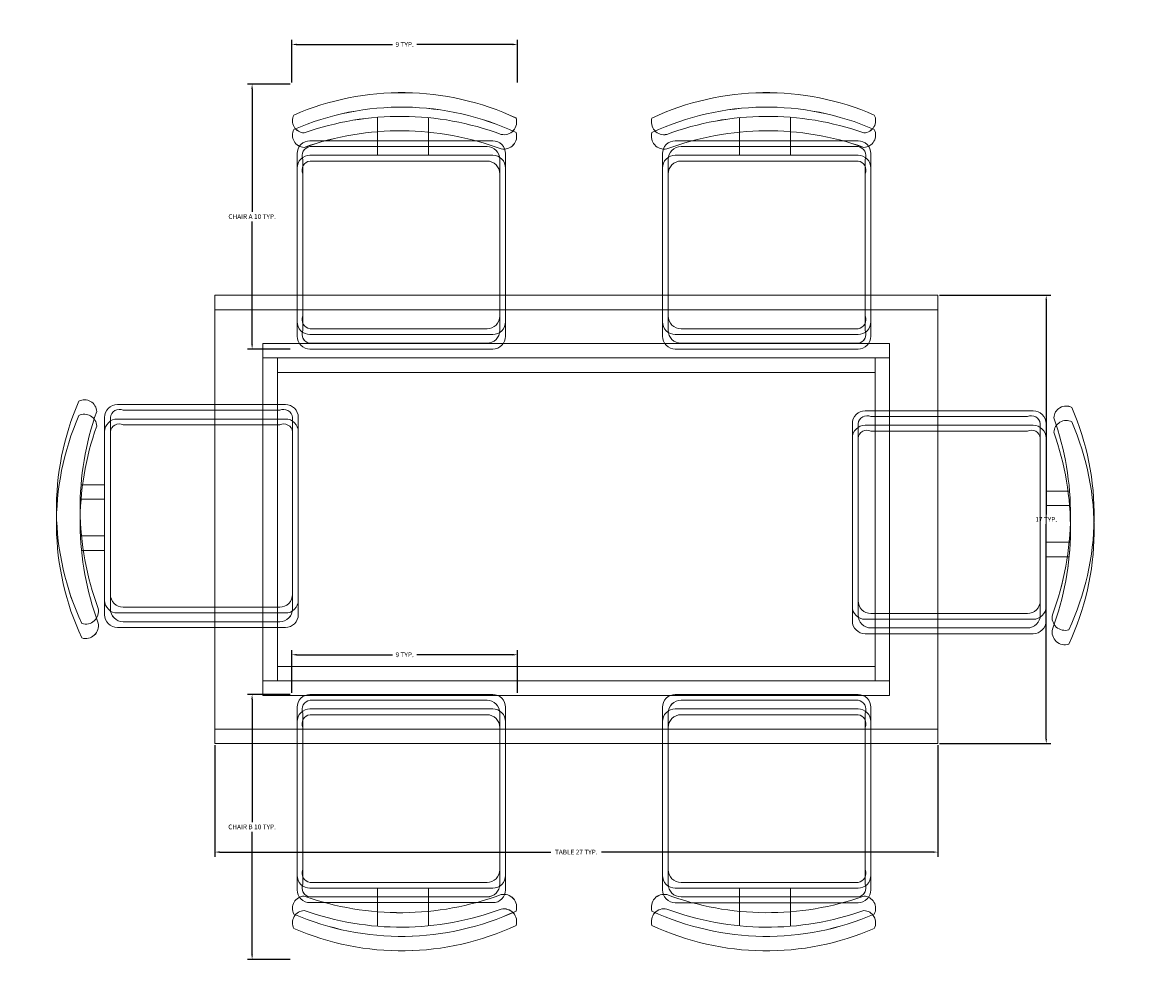
# Model space of a CAD drawing. Units: inches. Extents: x 2163 to 2982, y 1024 to 2288.
# Tile 14 of 22: x 2490 to 2532, y 1920 to 1957. Entities that reach past the tile are written whole.
import ezdxf

# ---------------------------------------------------------------- set-up
doc = ezdxf.new("R2010")
doc.units = ezdxf.units.IN
doc.layers.add('A-ANNO-DIMS', color=2, linetype='Continuous', lineweight=18)
doc.layers.add('A-FURN', color=8, linetype='Continuous', lineweight=13)
doc.styles.get("Standard").update_dxf_attribs({"font": 'arial.ttf'})
doc.dimstyles.get("Standard").update_dxf_attribs({"dimtxt": 0.18, "dimasz": 0.18, "dimexe": 0.18, "dimexo": 0.0625, "dimgap": 0.09, "dimtad": 0, "dimtih": 1, "dimtoh": 1, "dimdec": 4, "dimzin": 0, "dimdsep": 46, "dimtxsty": 'Standard', "dimcen": 0.09, "dimadec": 0, "dimazin": 0, "dimtfac": 1, "dimtdec": 4, "dimtofl": 0, "dimtmove": 0, "dimatfit": 3, "dimfxl": 1, "dimtolj": 1, "dimtzin": 0, "dimarcsym": 0})

# ---------------------------------------------------------------- blocks, each defined once
blk = doc.blocks.new('TABLE-DINING')
for points in [[(0, 17.017), (27.445, 17.017), (27.445, 0.549), (0, 0.549)], [(0, 17.017), (27.445, 17.017), (27.445, 0.549), (0, 0.549)], [(0, 17.016), (27.445, 17.016), (27.445, 0.549), (0, 0.549)], [(0, 17.016), (27.445, 17.016), (27.445, 0.549), (0, 0.549)], [(0, 16.468), (27.445, 16.468), (27.445, 0), (0, 0)], [(0, 16.468), (27.445, 16.468), (27.445, 0), (0, 0)], [(0, 16.467), (27.445, 16.467), (27.445, 0), (0, 0)], [(0, 16.467), (27.445, 16.467), (27.445, 0), (0, 0)], [(1.829, 15.187), (25.616, 15.187), (25.616, 2.379), (1.829, 2.379)], [(1.829, 15.187), (25.616, 15.187), (25.616, 2.379), (1.829, 2.379)], [(1.829, 15.187), (25.616, 15.187), (25.616, 2.379), (1.829, 2.379)], [(1.829, 15.187), (25.616, 15.187), (25.616, 2.379), (1.829, 2.379)], [(1.829, 14.638), (25.616, 14.638), (25.616, 1.83), (1.829, 1.83)], [(1.829, 14.638), (25.616, 14.638), (25.616, 1.83), (1.829, 1.83)], [(1.829, 14.638), (25.616, 14.638), (25.616, 1.83), (1.829, 1.83)], [(1.829, 14.638), (25.616, 14.638), (25.616, 1.83), (1.829, 1.83)], [(2.378, 14.638), (25.067, 14.638), (25.067, 2.928), (2.378, 2.928)], [(2.378, 14.638), (25.067, 14.638), (25.067, 2.927), (2.378, 2.927)], [(2.378, 14.638), (25.067, 14.638), (25.067, 2.928), (2.378, 2.928)], [(2.378, 14.638), (25.067, 14.638), (25.067, 2.927), (2.378, 2.927)], [(2.378, 14.089), (25.067, 14.089), (25.067, 2.379), (2.378, 2.379)], [(2.378, 14.089), (25.067, 14.089), (25.067, 2.379), (2.378, 2.379)], [(2.378, 14.089), (25.067, 14.089), (25.067, 2.379), (2.378, 2.379)], [(2.378, 14.089), (25.067, 14.089), (25.067, 2.379), (2.378, 2.379)]]:
    blk.add_lwpolyline(points, close=True)
blk = doc.blocks.new('CHAIR-DINING-A')
for points in [[(0.449, 8.202, -0.175809), (7.925, 8.145, 0.578392), (8.491, 8.768, 0.214524), (0.053, 8.881, 0.552014), (0.449, 8.202, -0.065079)], [(0.449, 8.201, -0.175809), (7.925, 8.145, 0.578392), (8.491, 8.767, 0.214524), (0.053, 8.881, 0.552014), (0.449, 8.201, -0.065079)], [(0.449, 8.202, -0.175809), (7.925, 8.145, 0.578392), (8.491, 8.768, 0.214524), (0.053, 8.881, 0.552014), (0.449, 8.202, -0.065079)], [(0.449, 8.201, -0.175809), (7.925, 8.145, 0.578392), (8.491, 8.767, 0.214524), (0.053, 8.881, 0.552014), (0.449, 8.201, -0.065079)], [(0.449, 7.653, -0.175809), (7.925, 7.596, 0.578392), (8.491, 8.219, 0.214524), (0.053, 8.332, 0.552014), (0.449, 7.653, -0.065079)], [(0.449, 7.652, -0.175809), (7.925, 7.596, 0.578392), (8.491, 8.218, 0.214524), (0.053, 8.332, 0.552014), (0.449, 7.652, -0.065079)], [(0.449, 7.653, -0.175809), (7.925, 7.596, 0.578392), (8.491, 8.219, 0.214524), (0.053, 8.332, 0.552014), (0.449, 7.653, -0.065079)], [(0.449, 7.652, -0.175809), (7.925, 7.596, 0.578392), (8.491, 8.218, 0.214524), (0.053, 8.332, 0.552014), (0.449, 7.652, -0.065079)], [(5.17, 7.902), (5.17, 8.779, -0.064759)], [(5.17, 7.901), (5.17, 8.779, -0.064759)], [(5.17, 7.902), (5.17, 8.779, -0.064759)], [(5.17, 7.901), (5.17, 8.779, -0.064759)], [(5.17, 7.353), (5.17, 8.23, -0.064759)], [(5.17, 7.352), (5.17, 8.23, -0.064759)], [(5.17, 7.353), (5.17, 8.23, -0.064759)], [(5.17, 7.352), (5.17, 8.23, -0.064759)], [(7.608, 7.902), (0.668, 7.902, 0.414214), (0.182, 7.416), (0.182, 1.035, 0.414214), (0.668, 0.549), (7.608, 0.549, 0.414214), (8.093, 1.035), (8.093, 7.416, 0.414214), (7.608, 7.902)], [(7.608, 7.902), (0.668, 7.902, 0.414214), (0.182, 7.416), (0.182, 1.035, 0.414214), (0.668, 0.549), (7.608, 0.549, 0.414214), (8.093, 1.035), (8.093, 7.416, 0.414214), (7.608, 7.902)], [(7.608, 7.901), (0.668, 7.901, 0.414214), (0.182, 7.416), (0.182, 1.035, 0.414214), (0.668, 0.549), (7.608, 0.549, 0.414214), (8.093, 1.035), (8.093, 7.416, 0.414214), (7.608, 7.901)], [(7.608, 7.901), (0.668, 7.901, 0.414214), (0.182, 7.416), (0.182, 1.035, 0.414214), (0.668, 0.549), (7.608, 0.549, 0.414214), (8.093, 1.035), (8.093, 7.416, 0.414214), (7.608, 7.901)], [(7.608, 7.353), (0.668, 7.353, 0.414214), (0.182, 6.867), (0.182, 0.486, 0.414214), (0.668, 0), (7.608, 0, 0.414214), (8.093, 0.486), (8.093, 6.867, 0.414214), (7.608, 7.353)], [(7.608, 7.353), (0.668, 7.353, 0.414214), (0.182, 6.867), (0.182, 0.486, 0.414214), (0.668, 0), (7.608, 0, 0.414214), (8.093, 0.486), (8.093, 6.867, 0.414214), (7.608, 7.353)], [(7.608, 7.352), (0.668, 7.352, 0.414214), (0.182, 6.867), (0.182, 0.486, 0.414214), (0.668, 0), (7.608, 0, 0.414214), (8.093, 0.486), (8.093, 6.867, 0.414214), (7.608, 7.352)], [(7.608, 7.352), (0.668, 7.352, 0.414214), (0.182, 6.867), (0.182, 0.486, 0.414214), (0.668, 0), (7.608, 0, 0.414214), (8.093, 0.486), (8.093, 6.867, 0.414214), (7.608, 7.352)]]:
    blk.add_lwpolyline(points, format="xyb")
for points in [[(3.227, 8.795), (3.227, 7.902)], [(3.227, 8.795), (3.227, 7.901)], [(3.227, 8.795), (3.227, 7.902)], [(3.227, 8.795), (3.227, 7.901)], [(3.227, 8.246), (3.227, 7.353)], [(3.227, 8.246), (3.227, 7.352)], [(3.227, 8.246), (3.227, 7.353)], [(3.227, 8.246), (3.227, 7.352)]]:
    blk.add_lwpolyline(points)
for points in [[(0.671, 7.683), (7.389, 7.683, -0.414214), (7.874, 7.197), (7.874, 1.254, -0.414214), (7.389, 0.768), (0.671, 0.768, -0.512069), (0.401, 1.254), (0.401, 7.197, -0.512069)], [(0.671, 7.683), (7.389, 7.683, -0.414214), (7.874, 7.197), (7.874, 1.254, -0.414214), (7.389, 0.768), (0.671, 0.768, -0.512069), (0.401, 1.254), (0.401, 7.197, -0.512069)], [(0.671, 7.682), (7.389, 7.682, -0.414214), (7.874, 7.197), (7.874, 1.253, -0.414214), (7.389, 0.768), (0.671, 0.768, -0.512069), (0.401, 1.253), (0.401, 7.197, -0.512069)], [(0.671, 7.682), (7.389, 7.682, -0.414214), (7.874, 7.197), (7.874, 1.253, -0.414214), (7.389, 0.768), (0.671, 0.768, -0.512069), (0.401, 1.253), (0.401, 7.197, -0.512069)], [(0.671, 7.134), (7.389, 7.134, -0.414214), (7.874, 6.648), (7.874, 0.705, -0.414214), (7.389, 0.219), (0.671, 0.219, -0.512069), (0.401, 0.705), (0.401, 6.648, -0.512069)], [(0.671, 7.134), (7.389, 7.134, -0.414214), (7.874, 6.648), (7.874, 0.704, -0.414214), (7.389, 0.219), (0.671, 0.219, -0.512069), (0.401, 0.704), (0.401, 6.648, -0.512069)], [(0.671, 7.134), (7.389, 7.134, -0.414214), (7.874, 6.648), (7.874, 0.705, -0.414214), (7.389, 0.219), (0.671, 0.219, -0.512069), (0.401, 0.705), (0.401, 6.648, -0.512069)], [(0.671, 7.134), (7.389, 7.134, -0.414214), (7.874, 6.648), (7.874, 0.704, -0.414214), (7.389, 0.219), (0.671, 0.219, -0.512069), (0.401, 0.704), (0.401, 6.648, -0.512069)]]:
    blk.add_lwpolyline(points, format="xyb", close=True)
blk = doc.blocks.new('CHAIR-DINING-B')
for points in [[(7.608, 2.377), (0.668, 2.377, -0.414214), (0.182, 2.862), (0.182, 9.243, -0.414214), (0.668, 9.729), (7.608, 9.729, -0.414214), (8.093, 9.243), (8.093, 2.862, -0.414214), (7.608, 2.377)], [(7.608, 2.376), (0.668, 2.376, -0.414214), (0.182, 2.862), (0.182, 9.243, -0.414214), (0.668, 9.729), (7.608, 9.729, -0.414214), (8.093, 9.243), (8.093, 2.862, -0.414214), (7.608, 2.376)], [(7.608, 2.377), (0.668, 2.377, -0.414214), (0.182, 2.862), (0.182, 9.243, -0.414214), (0.668, 9.729), (7.608, 9.729, -0.414214), (8.093, 9.243), (8.093, 2.862, -0.414214), (7.608, 2.377)], [(7.608, 2.376), (0.668, 2.376, -0.414214), (0.182, 2.862), (0.182, 9.243, -0.414214), (0.668, 9.729), (7.608, 9.729, -0.414214), (8.093, 9.243), (8.093, 2.862, -0.414214), (7.608, 2.376)], [(7.608, 1.828), (0.668, 1.828, -0.414214), (0.182, 2.313), (0.182, 8.695, -0.414214), (0.668, 9.18), (7.608, 9.18, -0.414214), (8.093, 8.695), (8.093, 2.313, -0.414214), (7.608, 1.828)], [(7.608, 1.828), (0.668, 1.828, -0.414214), (0.182, 2.313), (0.182, 8.694, -0.414214), (0.668, 9.18), (7.608, 9.18, -0.414214), (8.093, 8.694), (8.093, 2.313, -0.414214), (7.608, 1.828)], [(7.608, 1.828), (0.668, 1.828, -0.414214), (0.182, 2.313), (0.182, 8.695, -0.414214), (0.668, 9.18), (7.608, 9.18, -0.414214), (8.093, 8.695), (8.093, 2.313, -0.414214), (7.608, 1.828)], [(7.608, 1.828), (0.668, 1.828, -0.414214), (0.182, 2.313), (0.182, 8.694, -0.414214), (0.668, 9.18), (7.608, 9.18, -0.414214), (8.093, 8.694), (8.093, 2.313, -0.414214), (7.608, 1.828)], [(7.925, 2.133, -0.578392), (8.491, 1.511, -0.214524), (0.053, 1.397, -0.552014), (0.449, 2.077, 0.175809), (7.925, 2.133)], [(7.925, 2.133, -0.578392), (8.491, 1.511, -0.214524), (0.053, 1.397, -0.552014), (0.449, 2.077, 0.175809), (7.925, 2.133)], [(7.925, 2.133, -0.578392), (8.491, 1.51, -0.214524), (0.053, 1.397, -0.552014), (0.449, 2.076, 0.175809), (7.925, 2.133)], [(7.925, 2.133, -0.578392), (8.491, 1.51, -0.214524), (0.053, 1.397, -0.552014), (0.449, 2.076, 0.175809), (7.925, 2.133)], [(5.17, 2.377), (5.17, 1.499, 0.064759)], [(5.17, 2.377), (5.17, 1.499, 0.064759)], [(5.17, 2.376), (5.17, 1.499, 0.064759)], [(5.17, 2.376), (5.17, 1.499, 0.064759)], [(5.17, 1.828), (5.17, 0.95, 0.064759)], [(5.17, 1.828), (5.17, 0.95, 0.064759)], [(5.17, 1.828), (5.17, 0.95, 0.064759)], [(5.17, 1.828), (5.17, 0.95, 0.064759)], [(7.925, 1.584, -0.578392), (8.491, 0.962, -0.214524), (0.053, 0.848, -0.552014), (0.449, 1.528, 0.175809), (7.925, 1.584)], [(7.925, 1.584, -0.578392), (8.491, 0.962, -0.214524), (0.053, 0.848, -0.552014), (0.449, 1.528, 0.175809), (7.925, 1.584)], [(7.925, 1.584, -0.578392), (8.491, 0.961, -0.214524), (0.053, 0.848, -0.552014), (0.449, 1.528, 0.175809), (7.925, 1.584)], [(7.925, 1.584, -0.578392), (8.491, 0.961, -0.214524), (0.053, 0.848, -0.552014), (0.449, 1.528, 0.175809), (7.925, 1.584)]]:
    blk.add_lwpolyline(points, format="xyb")
for points in [[(0.671, 2.595), (7.389, 2.595, 0.414214), (7.874, 3.081), (7.874, 9.025, 0.414214), (7.389, 9.51), (0.671, 9.51, 0.512069), (0.401, 9.025), (0.401, 3.081, 0.512069)], [(0.671, 2.595), (7.389, 2.595, 0.414214), (7.874, 3.081), (7.874, 9.024, 0.414214), (7.389, 9.51), (0.671, 9.51, 0.512069), (0.401, 9.024), (0.401, 3.081, 0.512069)], [(0.671, 2.595), (7.389, 2.595, 0.414214), (7.874, 3.081), (7.874, 9.025, 0.414214), (7.389, 9.51), (0.671, 9.51, 0.512069), (0.401, 9.025), (0.401, 3.081, 0.512069)], [(0.671, 2.595), (7.389, 2.595, 0.414214), (7.874, 3.081), (7.874, 9.024, 0.414214), (7.389, 9.51), (0.671, 9.51, 0.512069), (0.401, 9.024), (0.401, 3.081, 0.512069)], [(0.671, 2.047), (7.389, 2.047, 0.414214), (7.874, 2.532), (7.874, 8.476, 0.414214), (7.389, 8.961), (0.671, 8.961, 0.512069), (0.401, 8.476), (0.401, 2.532, 0.512069)], [(0.671, 2.046), (7.389, 2.046, 0.414214), (7.874, 2.532), (7.874, 8.475, 0.414214), (7.389, 8.961), (0.671, 8.961, 0.512069), (0.401, 8.475), (0.401, 2.532, 0.512069)], [(0.671, 2.047), (7.389, 2.047, 0.414214), (7.874, 2.532), (7.874, 8.476, 0.414214), (7.389, 8.961), (0.671, 8.961, 0.512069), (0.401, 8.476), (0.401, 2.532, 0.512069)], [(0.671, 2.046), (7.389, 2.046, 0.414214), (7.874, 2.532), (7.874, 8.475, 0.414214), (7.389, 8.961), (0.671, 8.961, 0.512069), (0.401, 8.475), (0.401, 2.532, 0.512069)]]:
    blk.add_lwpolyline(points, format="xyb", close=True)
for points in [[(3.227, 1.483), (3.227, 2.377)], [(3.227, 1.483), (3.227, 2.377)], [(3.227, 1.483), (3.227, 2.376)], [(3.227, 1.483), (3.227, 2.376)], [(3.227, 0.934), (3.227, 1.828)], [(3.227, 0.934), (3.227, 1.828)], [(3.227, 0.934), (3.227, 1.828)], [(3.227, 0.934), (3.227, 1.828)]]:
    blk.add_lwpolyline(points)
blk = doc.blocks.new('*D19')
at = {"layer": 'A-ANNO-DIMS', "color": 0, "lineweight": -2, "transparency": 16777216}
for p, q in [((2500.314, 1954.461), (2498.688, 1954.461)), ((2498.868, 1954.281), (2498.868, 1949.618)), ((2498.868, 1944.589), (2498.868, 1949.252)), ((2500.314, 1944.409), (2498.688, 1944.409))]:
    blk.add_line(p, q, dxfattribs=at)
at = {"layer": 'A-ANNO-DIMS', "color": 0, "transparency": 16777216}
for points in [[(2498.838, 1954.281), (2498.898, 1954.281), (2498.868, 1954.461)], [(2498.838, 1944.589), (2498.898, 1944.589), (2498.868, 1944.409)]]:
    blk.add_solid(points, dxfattribs=at)
at = {"layer": 'Defpoints', "color": 0, "transparency": 16777216}
for p in [(2498.868, 1954.461), (2500.376, 1954.461), (2500.376, 1944.409)]:
    blk.add_point(p, dxfattribs=at)
at = {"layer": 'A-ANNO-DIMS', "color": 0, "transparency": 16777216, "insert": (2498.868, 1949.435), "char_height": 0.18, "attachment_point": 5}
blk.add_mtext('\\A1;CHAIR A 10 TYP.', dxfattribs=at)
blk = doc.blocks.new('*D20')
at = {"layer": 'A-ANNO-DIMS', "color": 0, "lineweight": -2, "transparency": 16777216}
for p, q in [((2500.376, 1954.523), (2500.376, 1956.148)), ((2500.556, 1955.968), (2504.2, 1955.968)), ((2508.761, 1955.968), (2505.117, 1955.968)), ((2508.941, 1954.523), (2508.941, 1956.148))]:
    blk.add_line(p, q, dxfattribs=at)
at = {"layer": 'A-ANNO-DIMS', "color": 0, "transparency": 16777216}
for points in [[(2500.556, 1955.998), (2500.556, 1955.938), (2500.376, 1955.968)], [(2508.761, 1955.998), (2508.761, 1955.938), (2508.941, 1955.968)]]:
    blk.add_solid(points, dxfattribs=at)
at = {"layer": 'Defpoints', "color": 0, "transparency": 16777216}
for p in [(2508.941, 1955.968), (2500.376, 1954.461), (2508.941, 1954.461)]:
    blk.add_point(p, dxfattribs=at)
at = {"layer": 'A-ANNO-DIMS', "color": 0, "transparency": 16777216, "insert": (2504.659, 1955.968), "char_height": 0.18, "attachment_point": 5}
blk.add_mtext('\\A1;9 TYP.', dxfattribs=at)
blk = doc.blocks.new('*D21')
at = {"layer": 'A-ANNO-DIMS', "color": 0, "lineweight": -2, "transparency": 16777216}
for p, q in [((2500.314, 1931.297), (2498.688, 1931.297)), ((2498.868, 1931.117), (2498.868, 1926.454)), ((2498.868, 1921.425), (2498.868, 1926.088)), ((2500.314, 1921.245), (2498.688, 1921.245))]:
    blk.add_line(p, q, dxfattribs=at)
at = {"layer": 'A-ANNO-DIMS', "color": 0, "transparency": 16777216}
for points in [[(2498.838, 1931.117), (2498.898, 1931.117), (2498.868, 1931.297)], [(2498.838, 1921.425), (2498.898, 1921.425), (2498.868, 1921.245)]]:
    blk.add_solid(points, dxfattribs=at)
at = {"layer": 'Defpoints', "color": 0, "transparency": 16777216}
for p in [(2498.868, 1931.297), (2500.376, 1931.297), (2500.376, 1921.245)]:
    blk.add_point(p, dxfattribs=at)
at = {"layer": 'A-ANNO-DIMS', "color": 0, "transparency": 16777216, "insert": (2498.868, 1926.271), "char_height": 0.18, "attachment_point": 5}
blk.add_mtext('\\A1;CHAIR B 10 TYP.', dxfattribs=at)
blk = doc.blocks.new('*D22')
at = {"layer": 'A-ANNO-DIMS', "color": 0, "lineweight": -2, "transparency": 16777216}
for p, q in [((2500.376, 1931.359), (2500.376, 1932.985)), ((2500.556, 1932.805), (2504.2, 1932.805)), ((2508.761, 1932.805), (2505.117, 1932.805)), ((2508.941, 1931.359), (2508.941, 1932.985))]:
    blk.add_line(p, q, dxfattribs=at)
at = {"layer": 'A-ANNO-DIMS', "color": 0, "transparency": 16777216}
for points in [[(2500.556, 1932.835), (2500.556, 1932.775), (2500.376, 1932.805)], [(2508.761, 1932.835), (2508.761, 1932.775), (2508.941, 1932.805)]]:
    blk.add_solid(points, dxfattribs=at)
at = {"layer": 'Defpoints', "color": 0, "transparency": 16777216}
for p in [(2508.941, 1932.805), (2500.376, 1931.297), (2508.941, 1931.297)]:
    blk.add_point(p, dxfattribs=at)
at = {"layer": 'A-ANNO-DIMS', "color": 0, "transparency": 16777216, "insert": (2504.659, 1932.805), "char_height": 0.18, "attachment_point": 5}
blk.add_mtext('\\A1;9 TYP.', dxfattribs=at)
blk = doc.blocks.new('*D23')
at = {"layer": 'A-ANNO-DIMS', "color": 0, "lineweight": -2, "transparency": 16777216}
for p, q in [((2497.452, 1929.37), (2497.452, 1925.136)), ((2524.897, 1929.37), (2524.897, 1925.136)), ((2497.632, 1925.316), (2510.211, 1925.316)), ((2524.717, 1925.316), (2512.138, 1925.316))]:
    blk.add_line(p, q, dxfattribs=at)
at = {"layer": 'A-ANNO-DIMS', "color": 0, "transparency": 16777216}
for points in [[(2497.632, 1925.346), (2497.632, 1925.286), (2497.452, 1925.316)], [(2524.717, 1925.346), (2524.717, 1925.286), (2524.897, 1925.316)]]:
    blk.add_solid(points, dxfattribs=at)
at = {"layer": 'Defpoints', "color": 0, "transparency": 16777216}
for p in [(2497.452, 1929.433), (2524.897, 1929.433), (2524.897, 1925.316)]:
    blk.add_point(p, dxfattribs=at)
at = {"layer": 'A-ANNO-DIMS', "color": 0, "transparency": 16777216, "insert": (2511.174, 1925.316), "char_height": 0.18, "attachment_point": 5}
blk.add_mtext('\\A1;TABLE 27 TYP.', dxfattribs=at)
blk = doc.blocks.new('*D24')
at = {"layer": 'A-ANNO-DIMS', "color": 0, "lineweight": -2, "transparency": 16777216}
for p, q in [((2524.96, 1946.45), (2529.194, 1946.45)), ((2529.014, 1946.27), (2529.014, 1938.122)), ((2529.014, 1929.613), (2529.014, 1937.761)), ((2524.96, 1929.433), (2529.194, 1929.433))]:
    blk.add_line(p, q, dxfattribs=at)
at = {"layer": 'A-ANNO-DIMS', "color": 0, "transparency": 16777216}
for points in [[(2528.984, 1946.27), (2529.044, 1946.27), (2529.014, 1946.45)], [(2528.984, 1929.613), (2529.044, 1929.613), (2529.014, 1929.433)]]:
    blk.add_solid(points, dxfattribs=at)
at = {"layer": 'Defpoints', "color": 0, "transparency": 16777216}
for p in [(2524.897, 1946.45), (2529.014, 1946.45), (2524.897, 1929.433)]:
    blk.add_point(p, dxfattribs=at)
at = {"layer": 'A-ANNO-DIMS', "color": 0, "transparency": 16777216, "insert": (2529.014, 1937.941), "char_height": 0.18, "attachment_point": 5}
blk.add_mtext('\\A1;17 TYP.', dxfattribs=at)
blk = doc.blocks.new('*D29')
at = {"layer": 'A-ANNO-DIMS', "color": 0, "lineweight": -2, "transparency": 16777216}
for p, q in [((2285.339, 1738.831), (2285.339, 2288.099)), ((2867.339, 2229.331), (2867.339, 2288.099)), ((2285.519, 2287.919), (2576.051, 2287.919)), ((2867.159, 2287.919), (2576.627, 2287.919))]:
    blk.add_line(p, q, dxfattribs=at)
at = {"layer": 'A-ANNO-DIMS', "color": 0, "transparency": 16777216}
for points in [[(2285.519, 2287.949), (2285.519, 2287.889), (2285.339, 2287.919)], [(2867.159, 2287.949), (2867.159, 2287.889), (2867.339, 2287.919)]]:
    blk.add_solid(points, dxfattribs=at)
at = {"layer": 'Defpoints', "color": 0, "transparency": 16777216}
for p in [(2867.339, 2287.919), (2867.339, 2229.269), (2285.339, 1738.769)]:
    blk.add_point(p, dxfattribs=at)
at = {"layer": 'A-ANNO-DIMS', "color": 0, "transparency": 16777216, "insert": (2576.339, 2287.919), "char_height": 0.18, "attachment_point": 5}
blk.add_mtext('\\A1;582', dxfattribs=at)

msp = doc.modelspace()

# ---------------------------------------------------------------- linework, layer by layer
at = {"layer": 'A-FURN'}
for points in [[(2514.6151, 1952.5539, -0.5783921), (2514.0487, 1953.1766, -0.2145244), (2522.4869, 1953.2899, -0.552014), (2522.0905, 1952.6105, 0.1758092), (2514.6151, 1952.5539)], [(2514.6151, 1952.5539, -0.5783921), (2514.0487, 1953.1766, -0.2145244), (2522.4869, 1953.2899, -0.552014), (2522.0905, 1952.6105, 0.1758092), (2514.6151, 1952.5539)], [(2514.6151, 1952.5536, -0.5783921), (2514.0487, 1953.1764, -0.2145244), (2522.4869, 1953.2896, -0.552014), (2522.0905, 1952.6103, 0.1758092), (2514.6151, 1952.5536)], [(2514.6151, 1952.5536, -0.5783921), (2514.0487, 1953.1764, -0.2145244), (2522.4869, 1953.2896, -0.552014), (2522.0905, 1952.6103, 0.1758092), (2514.6151, 1952.5536)], [(2514.6151, 1952.005, -0.5783921), (2514.0487, 1952.6277, -0.2145244), (2522.4869, 1952.741, -0.552014), (2522.0905, 1952.0616, 0.1758092), (2514.6151, 1952.005)], [(2514.6151, 1952.005, -0.5783921), (2514.0487, 1952.6277, -0.2145244), (2522.4869, 1952.741, -0.552014), (2522.0905, 1952.0616, 0.1758092), (2514.6151, 1952.005)], [(2514.6151, 1952.0047, -0.5783921), (2514.0487, 1952.6274, -0.2145244), (2522.4869, 1952.7407, -0.552014), (2522.0905, 1952.0613, 0.1758092), (2514.6151, 1952.0047)], [(2514.6151, 1952.0047, -0.5783921), (2514.0487, 1952.6274, -0.2145244), (2522.4869, 1952.7407, -0.552014), (2522.0905, 1952.0613, 0.1758092), (2514.6151, 1952.0047)], [(2517.3699, 1952.3105), (2517.3699, 1953.1882, 0.0647586)], [(2517.3699, 1952.3105), (2517.3699, 1953.1882, 0.0647586)], [(2517.3699, 1952.3102), (2517.3699, 1953.1879, 0.0647586)], [(2517.3699, 1952.3102), (2517.3699, 1953.1879, 0.0647586)], [(2517.3699, 1951.7616), (2517.3699, 1952.6393, 0.0647586)], [(2517.3699, 1951.7616), (2517.3699, 1952.6393, 0.0647586)], [(2517.3699, 1951.7613), (2517.3699, 1952.639, 0.0647586)], [(2517.3699, 1951.7613), (2517.3699, 1952.639, 0.0647586)], [(2521.8721, 1952.3105, -0.4142136), (2522.3577, 1951.825), (2522.3577, 1945.4438, -0.4142136), (2521.8721, 1944.9583), (2514.9322, 1944.9583, -0.4142136), (2514.4467, 1945.4438), (2514.4467, 1951.825, -0.4142136), (2514.9322, 1952.3105), (2521.8721, 1952.3105)], [(2521.8721, 1952.3105, -0.4142136), (2522.3577, 1951.825), (2522.3577, 1945.4438, -0.4142136), (2521.8721, 1944.9583), (2514.9322, 1944.9583, -0.4142136), (2514.4467, 1945.4438), (2514.4467, 1951.825, -0.4142136), (2514.9322, 1952.3105), (2521.8721, 1952.3105)], [(2521.8722, 1952.3102, -0.4142136), (2522.3577, 1951.8247), (2522.3577, 1945.4436, -0.4142136), (2521.8722, 1944.958), (2514.9322, 1944.958, -0.4142136), (2514.4467, 1945.4436), (2514.4467, 1951.8247, -0.4142136), (2514.9322, 1952.3102), (2521.8722, 1952.3102)], [(2521.8722, 1952.3102, -0.4142136), (2522.3577, 1951.8247), (2522.3577, 1945.4436, -0.4142136), (2521.8722, 1944.958), (2514.9322, 1944.958, -0.4142136), (2514.4467, 1945.4436), (2514.4467, 1951.8247, -0.4142136), (2514.9322, 1952.3102), (2521.8722, 1952.3102)], [(2521.8721, 1951.7616, -0.4142136), (2522.3577, 1951.2761), (2522.3577, 1944.8949, -0.4142136), (2521.8721, 1944.4094), (2514.9322, 1944.4094, -0.4142136), (2514.4467, 1944.8949), (2514.4467, 1951.2761, -0.4142136), (2514.9322, 1951.7616), (2521.8721, 1951.7616)], [(2521.8721, 1951.7616, -0.4142136), (2522.3577, 1951.2761), (2522.3577, 1944.8949, -0.4142136), (2521.8721, 1944.4094), (2514.9322, 1944.4094, -0.4142136), (2514.4467, 1944.8949), (2514.4467, 1951.2761, -0.4142136), (2514.9322, 1951.7616), (2521.8721, 1951.7616)], [(2521.8722, 1951.7613, -0.4142136), (2522.3577, 1951.2758), (2522.3577, 1944.8946, -0.4142136), (2521.8722, 1944.4091), (2514.9322, 1944.4091, -0.4142136), (2514.4467, 1944.8946), (2514.4467, 1951.2758, -0.4142136), (2514.9322, 1951.7613), (2521.8722, 1951.7613)], [(2521.8722, 1951.7613, -0.4142136), (2522.3577, 1951.2758), (2522.3577, 1944.8946, -0.4142136), (2521.8722, 1944.4091), (2514.9322, 1944.4091, -0.4142136), (2514.4467, 1944.8946), (2514.4467, 1951.2758, -0.4142136), (2514.9322, 1951.7613), (2521.8722, 1951.7613)], [(2493.0255, 1934.5585, -0.5783921), (2492.4028, 1933.9922, -0.2145244), (2492.2896, 1942.4304, -0.552014), (2492.9689, 1942.0339, 0.1758094), (2493.0255, 1934.5585)], [(2493.0255, 1934.5585, -0.5783921), (2492.4028, 1933.9922, -0.2145244), (2492.2896, 1942.4304, -0.552014), (2492.9689, 1942.0339, 0.1758094), (2493.0255, 1934.5585)], [(2493.0255, 1934.5582, -0.5783921), (2492.4028, 1933.9919, -0.2145244), (2492.2896, 1942.4301, -0.552014), (2492.9689, 1942.0336, 0.1758094), (2493.0255, 1934.5582)], [(2493.0255, 1934.5582, -0.5783921), (2492.4028, 1933.9919, -0.2145244), (2492.2896, 1942.4301, -0.552014), (2492.9689, 1942.0336, 0.1758094), (2493.0255, 1934.5582)], [(2493.2689, 1941.8156, -0.4142136), (2493.7545, 1942.3011), (2500.1356, 1942.3011, -0.4142136), (2500.6211, 1941.8156), (2500.6211, 1934.8756, -0.4142136), (2500.1356, 1934.3901), (2493.7545, 1934.3901, -0.4142136), (2493.2689, 1934.8756), (2493.2689, 1941.8156)], [(2493.2689, 1941.8156, -0.4142136), (2493.7545, 1942.3011), (2500.1356, 1942.3011, -0.4142136), (2500.6211, 1941.8156), (2500.6211, 1934.8756, -0.4142136), (2500.1356, 1934.3901), (2493.7545, 1934.3901, -0.4142136), (2493.2689, 1934.8756), (2493.2689, 1941.8156)], [(2493.269, 1941.8153, -0.4142136), (2493.7545, 1942.3008), (2500.1356, 1942.3008, -0.4142136), (2500.6211, 1941.8153), (2500.6211, 1934.8754, -0.4142136), (2500.1356, 1934.3898), (2493.7545, 1934.3898, -0.4142136), (2493.269, 1934.8754), (2493.269, 1941.8153)], [(2493.269, 1941.8153, -0.4142136), (2493.7545, 1942.3008), (2500.1356, 1942.3008, -0.4142136), (2500.6211, 1941.8153), (2500.6211, 1934.8754, -0.4142136), (2500.1356, 1934.3898), (2493.7545, 1934.3898, -0.4142136), (2493.269, 1934.8754), (2493.269, 1941.8153)], [(2493.0255, 1934.0096, -0.5783921), (2492.4028, 1933.4433, -0.2145244), (2492.2896, 1941.8814, -0.552014), (2492.9689, 1941.485, 0.1758094), (2493.0255, 1934.0096)], [(2493.0255, 1934.0096, -0.5783921), (2492.4028, 1933.4433, -0.2145244), (2492.2896, 1941.8814, -0.552014), (2492.9689, 1941.485, 0.1758094), (2493.0255, 1934.0096)], [(2493.0255, 1934.0093, -0.5783921), (2492.4028, 1933.443, -0.2145244), (2492.2896, 1941.8812, -0.552014), (2492.9689, 1941.4847, 0.1758094), (2493.0255, 1934.0093)], [(2493.0255, 1934.0093, -0.5783921), (2492.4028, 1933.443, -0.2145244), (2492.2896, 1941.8812, -0.552014), (2492.9689, 1941.4847, 0.1758094), (2493.0255, 1934.0093)], [(2529.0064, 1941.5779, 0.4142136), (2528.5209, 1942.0634), (2522.1397, 1942.0634, 0.4142136), (2521.6542, 1941.5779), (2521.6542, 1934.638, 0.4142136), (2522.1397, 1934.1524), (2528.5209, 1934.1524, 0.4142136), (2529.0064, 1934.638), (2529.0064, 1941.5779)], [(2529.0064, 1941.5779, 0.4142136), (2528.5209, 1942.0634), (2522.1397, 1942.0634, 0.4142136), (2521.6542, 1941.5779), (2521.6542, 1934.638, 0.4142136), (2522.1397, 1934.1524), (2528.5209, 1934.1524, 0.4142136), (2529.0064, 1934.638), (2529.0064, 1941.5779)], [(2529.0064, 1941.5776, 0.4142136), (2528.5209, 1942.0631), (2522.1397, 1942.0631, 0.4142136), (2521.6542, 1941.5776), (2521.6542, 1934.6377, 0.4142136), (2522.1397, 1934.1522), (2528.5209, 1934.1522, 0.4142136), (2529.0064, 1934.6377), (2529.0064, 1941.5776)], [(2529.0064, 1941.5776, 0.4142136), (2528.5209, 1942.0631), (2522.1397, 1942.0631, 0.4142136), (2521.6542, 1941.5776), (2521.6542, 1934.6377, 0.4142136), (2522.1397, 1934.1522), (2528.5209, 1934.1522, 0.4142136), (2529.0064, 1934.6377), (2529.0064, 1941.5776)], [(2529.3064, 1941.7962, -0.1758092), (2529.2498, 1934.3208, 0.5783921), (2529.8725, 1933.7545, 0.2145244), (2529.9858, 1942.1927, 0.552014), (2529.3064, 1941.7963, -0.065079)], [(2529.3064, 1941.7962, -0.1758092), (2529.2498, 1934.3208, 0.5783921), (2529.8725, 1933.7545, 0.2145244), (2529.9858, 1942.1927, 0.552014), (2529.3064, 1941.7963, -0.065079)], [(2529.3064, 1941.796, -0.1758092), (2529.2498, 1934.3205, 0.5783921), (2529.8725, 1933.7542, 0.2145244), (2529.9858, 1942.1924, 0.552014), (2529.3064, 1941.796, -0.065079)], [(2529.3064, 1941.796, -0.1758092), (2529.2498, 1934.3205, 0.5783921), (2529.8725, 1933.7542, 0.2145244), (2529.9858, 1942.1924, 0.552014), (2529.3064, 1941.796, -0.065079)], [(2493.2689, 1941.2667, -0.4142136), (2493.7545, 1941.7522), (2500.1356, 1941.7522, -0.4142136), (2500.6211, 1941.2667), (2500.6211, 1934.3267, -0.4142136), (2500.1356, 1933.8412), (2493.7545, 1933.8412, -0.4142136), (2493.2689, 1934.3267), (2493.2689, 1941.2667)], [(2493.2689, 1941.2667, -0.4142136), (2493.7545, 1941.7522), (2500.1356, 1941.7522, -0.4142136), (2500.6211, 1941.2667), (2500.6211, 1934.3267, -0.4142136), (2500.1356, 1933.8412), (2493.7545, 1933.8412, -0.4142136), (2493.2689, 1934.3267), (2493.2689, 1941.2667)], [(2493.269, 1941.2664, -0.4142136), (2493.7545, 1941.7519), (2500.1356, 1941.7519, -0.4142136), (2500.6211, 1941.2664), (2500.6211, 1934.3264, -0.4142136), (2500.1356, 1933.8409), (2493.7545, 1933.8409, -0.4142136), (2493.269, 1934.3264), (2493.269, 1941.2664)], [(2493.269, 1941.2664, -0.4142136), (2493.7545, 1941.7519), (2500.1356, 1941.7519, -0.4142136), (2500.6211, 1941.2664), (2500.6211, 1934.3264, -0.4142136), (2500.1356, 1933.8409), (2493.7545, 1933.8409, -0.4142136), (2493.269, 1934.3264), (2493.269, 1941.2664)], [(2529.0064, 1941.029, 0.4142136), (2528.5209, 1941.5145), (2522.1397, 1941.5145, 0.4142136), (2521.6542, 1941.029), (2521.6542, 1934.0891, 0.4142136), (2522.1397, 1933.6035), (2528.5209, 1933.6035, 0.4142136), (2529.0064, 1934.0891), (2529.0064, 1941.029)], [(2529.0064, 1941.029, 0.4142136), (2528.5209, 1941.5145), (2522.1397, 1941.5145, 0.4142136), (2521.6542, 1941.029), (2521.6542, 1934.0891, 0.4142136), (2522.1397, 1933.6035), (2528.5209, 1933.6035, 0.4142136), (2529.0064, 1934.0891), (2529.0064, 1941.029)], [(2529.0064, 1941.0287, 0.4142136), (2528.5209, 1941.5142), (2522.1397, 1941.5142, 0.4142136), (2521.6542, 1941.0287), (2521.6542, 1934.0888, 0.4142136), (2522.1397, 1933.6032), (2528.5209, 1933.6032, 0.4142136), (2529.0064, 1934.0888), (2529.0064, 1941.0287)], [(2529.0064, 1941.0287, 0.4142136), (2528.5209, 1941.5142), (2522.1397, 1941.5142, 0.4142136), (2521.6542, 1941.0287), (2521.6542, 1934.0888, 0.4142136), (2522.1397, 1933.6032), (2528.5209, 1933.6032, 0.4142136), (2529.0064, 1934.0888), (2529.0064, 1941.0287)], [(2529.3064, 1941.2473, -0.1758092), (2529.2498, 1933.7719, 0.5783921), (2529.8725, 1933.2056, 0.2145244), (2529.9858, 1941.6438, 0.552014), (2529.3064, 1941.2473, -0.065079)], [(2529.3064, 1941.2473, -0.1758092), (2529.2498, 1933.7719, 0.5783921), (2529.8725, 1933.2056, 0.2145244), (2529.9858, 1941.6438, 0.552014), (2529.3064, 1941.2473, -0.065079)], [(2529.3064, 1941.247, -0.1758092), (2529.2498, 1933.7716, 0.5783921), (2529.8725, 1933.2053, 0.2145244), (2529.9858, 1941.6435, 0.552014), (2529.3064, 1941.247, -0.065079)], [(2529.3064, 1941.247, -0.1758092), (2529.2498, 1933.7716, 0.5783921), (2529.8725, 1933.2053, 0.2145244), (2529.9858, 1941.6435, 0.552014), (2529.3064, 1941.247, -0.065079)], [(2493.2689, 1937.3133), (2492.3912, 1937.3133, 0.0647586)], [(2493.2689, 1937.3133), (2492.3912, 1937.3133, 0.0647586)], [(2493.269, 1937.313), (2492.3913, 1937.313, 0.0647586)], [(2493.269, 1937.313), (2492.3913, 1937.313, 0.0647586)], [(2529.0064, 1937.0756), (2529.8841, 1937.0756, -0.0647586)], [(2529.0064, 1937.0756), (2529.8841, 1937.0756, -0.0647586)], [(2529.0064, 1937.0753), (2529.8841, 1937.0753, -0.0647586)], [(2529.0064, 1937.0753), (2529.8841, 1937.0753, -0.0647586)], [(2493.2689, 1936.7644), (2492.3912, 1936.7644, 0.0647586)], [(2493.2689, 1936.7644), (2492.3912, 1936.7644, 0.0647586)], [(2493.269, 1936.7641), (2492.3913, 1936.7641, 0.0647586)], [(2493.269, 1936.7641), (2492.3913, 1936.7641, 0.0647586)], [(2529.0064, 1936.5267), (2529.8841, 1936.5267, -0.0647586)], [(2529.0064, 1936.5267), (2529.8841, 1936.5267, -0.0647586)], [(2529.0064, 1936.5264), (2529.8841, 1936.5264, -0.0647586)], [(2529.0064, 1936.5264), (2529.8841, 1936.5264, -0.0647586)], [(2521.8721, 1923.9448, 0.4142136), (2522.3577, 1924.4303), (2522.3577, 1930.8114, 0.4142136), (2521.8721, 1931.297), (2514.9322, 1931.297, 0.4142136), (2514.4467, 1930.8114), (2514.4467, 1924.4303, 0.4142136), (2514.9322, 1923.9448), (2521.8721, 1923.9448)], [(2521.8721, 1923.9448, 0.4142136), (2522.3577, 1924.4303), (2522.3577, 1930.8114, 0.4142136), (2521.8721, 1931.297), (2514.9322, 1931.297, 0.4142136), (2514.4467, 1930.8114), (2514.4467, 1924.4303, 0.4142136), (2514.9322, 1923.9448), (2521.8721, 1923.9448)], [(2521.8722, 1923.9445, 0.4142136), (2522.3577, 1924.43), (2522.3577, 1930.8111, 0.4142136), (2521.8722, 1931.2967), (2514.9322, 1931.2967, 0.4142136), (2514.4467, 1930.8111), (2514.4467, 1924.43, 0.4142136), (2514.9322, 1923.9445), (2521.8722, 1923.9445)], [(2521.8722, 1923.9445, 0.4142136), (2522.3577, 1924.43), (2522.3577, 1930.8111, 0.4142136), (2521.8722, 1931.2967), (2514.9322, 1931.2967, 0.4142136), (2514.4467, 1930.8111), (2514.4467, 1924.43, 0.4142136), (2514.9322, 1923.9445), (2521.8722, 1923.9445)], [(2521.8721, 1923.3958, 0.4142136), (2522.3577, 1923.8814), (2522.3577, 1930.2625, 0.4142136), (2521.8721, 1930.748), (2514.9322, 1930.748, 0.4142136), (2514.4467, 1930.2625), (2514.4467, 1923.8814, 0.4142136), (2514.9322, 1923.3958), (2521.8721, 1923.3958)], [(2521.8721, 1923.3958, 0.4142136), (2522.3577, 1923.8814), (2522.3577, 1930.2625, 0.4142136), (2521.8721, 1930.748), (2514.9322, 1930.748, 0.4142136), (2514.4467, 1930.2625), (2514.4467, 1923.8814, 0.4142136), (2514.9322, 1923.3958), (2521.8721, 1923.3958)], [(2521.8722, 1923.3956, 0.4142136), (2522.3577, 1923.8811), (2522.3577, 1930.2622, 0.4142136), (2521.8722, 1930.7478), (2514.9322, 1930.7478, 0.4142136), (2514.4467, 1930.2622), (2514.4467, 1923.8811, 0.4142136), (2514.9322, 1923.3956), (2521.8722, 1923.3956)], [(2521.8722, 1923.3956, 0.4142136), (2522.3577, 1923.8811), (2522.3577, 1930.2622, 0.4142136), (2521.8722, 1930.7478), (2514.9322, 1930.7478, 0.4142136), (2514.4467, 1930.2622), (2514.4467, 1923.8811, 0.4142136), (2514.9322, 1923.3956), (2521.8722, 1923.3956)], [(2517.3699, 1923.9448), (2517.3699, 1923.0671, -0.0647586)], [(2517.3699, 1923.9448), (2517.3699, 1923.0671, -0.0647586)], [(2517.3699, 1923.9445), (2517.3699, 1923.0668, -0.0647586)], [(2517.3699, 1923.9445), (2517.3699, 1923.0668, -0.0647586)], [(2522.0905, 1923.6447, -0.1758093), (2514.6151, 1923.7013, 0.5783921), (2514.0487, 1923.0786, 0.2145244), (2522.4869, 1922.9654, 0.552014), (2522.0905, 1923.6447, -0.065079)], [(2522.0905, 1923.6447, -0.1758093), (2514.6151, 1923.7013, 0.5783921), (2514.0487, 1923.0786, 0.2145244), (2522.4869, 1922.9654, 0.552014), (2522.0905, 1923.6447, -0.065079)], [(2522.0905, 1923.6444, -0.1758093), (2514.6151, 1923.7011, 0.5783921), (2514.0487, 1923.0783, 0.2145244), (2522.4869, 1922.9651, 0.552014), (2522.0905, 1923.6444, -0.065079)], [(2522.0905, 1923.6444, -0.1758093), (2514.6151, 1923.7011, 0.5783921), (2514.0487, 1923.0783, 0.2145244), (2522.4869, 1922.9651, 0.552014), (2522.0905, 1923.6444, -0.065079)], [(2517.3699, 1923.3958), (2517.3699, 1922.5182, -0.0647586)], [(2517.3699, 1923.3958), (2517.3699, 1922.5182, -0.0647586)], [(2517.3699, 1923.3956), (2517.3699, 1922.5179, -0.0647586)], [(2517.3699, 1923.3956), (2517.3699, 1922.5179, -0.0647586)], [(2522.0905, 1923.0958, -0.1758093), (2514.6151, 1923.1524, 0.5783921), (2514.0487, 1922.5297, 0.2145244), (2522.4869, 1922.4165, 0.552014), (2522.0905, 1923.0958, -0.065079)], [(2522.0905, 1923.0958, -0.1758093), (2514.6151, 1923.1524, 0.5783921), (2514.0487, 1922.5297, 0.2145244), (2522.4869, 1922.4165, 0.552014), (2522.0905, 1923.0958, -0.065079)], [(2522.0905, 1923.0955, -0.1758093), (2514.6151, 1923.1521, 0.5783921), (2514.0487, 1922.5294, 0.2145244), (2522.4869, 1922.4162, 0.552014), (2522.0905, 1923.0955, -0.065079)], [(2522.0905, 1923.0955, -0.1758093), (2514.6151, 1923.1521, 0.5783921), (2514.0487, 1922.5294, 0.2145244), (2522.4869, 1922.4162, 0.552014), (2522.0905, 1923.0955, -0.065079)]]:
    msp.add_lwpolyline(points, format="xyb", dxfattribs=at)
for points in [[(2519.3125, 1953.2042), (2519.3125, 1952.3105)], [(2519.3125, 1953.2042), (2519.3125, 1952.3105)], [(2519.3125, 1953.2039), (2519.3125, 1952.3102)], [(2519.3125, 1953.2039), (2519.3125, 1952.3102)], [(2519.3125, 1952.6552), (2519.3125, 1951.7616)], [(2519.3125, 1952.6552), (2519.3125, 1951.7616)], [(2519.3125, 1952.6549), (2519.3125, 1951.7613)], [(2519.3125, 1952.6549), (2519.3125, 1951.7613)], [(2492.3753, 1939.2559), (2493.2689, 1939.2559)], [(2492.3753, 1939.2559), (2493.2689, 1939.2559)], [(2492.3753, 1939.2556), (2493.269, 1939.2556)], [(2492.3753, 1939.2556), (2493.269, 1939.2556)], [(2529.9, 1939.0182), (2529.0064, 1939.0182)], [(2529.9, 1939.0182), (2529.0064, 1939.0182)], [(2529.9001, 1939.0179), (2529.0064, 1939.0179)], [(2529.9001, 1939.0179), (2529.0064, 1939.0179)], [(2492.3753, 1938.707), (2493.2689, 1938.707)], [(2492.3753, 1938.707), (2493.2689, 1938.707)], [(2492.3753, 1938.7067), (2493.269, 1938.7067)], [(2492.3753, 1938.7067), (2493.269, 1938.7067)], [(2529.9, 1938.4693), (2529.0064, 1938.4693)], [(2529.9, 1938.4693), (2529.0064, 1938.4693)], [(2529.9001, 1938.469), (2529.0064, 1938.469)], [(2529.9001, 1938.469), (2529.0064, 1938.469)], [(2519.3125, 1923.0511), (2519.3125, 1923.9448)], [(2519.3125, 1923.0511), (2519.3125, 1923.9448)], [(2519.3125, 1923.0508), (2519.3125, 1923.9445)], [(2519.3125, 1923.0508), (2519.3125, 1923.9445)], [(2519.3125, 1922.5022), (2519.3125, 1923.3958)], [(2519.3125, 1922.5022), (2519.3125, 1923.3958)], [(2519.3125, 1922.5019), (2519.3125, 1923.3956)], [(2519.3125, 1922.5019), (2519.3125, 1923.3956)]]:
    msp.add_lwpolyline(points, dxfattribs=at)
for points in [[(2521.8692, 1952.0918), (2515.1509, 1952.0918, 0.4142136), (2514.6654, 1951.6063), (2514.6654, 1945.6626, 0.4142136), (2515.1509, 1945.177), (2521.8692, 1945.177, 0.5120695), (2522.1389, 1945.6626), (2522.1389, 1951.6063, 0.5120695)], [(2521.8692, 1952.0918), (2515.1509, 1952.0918, 0.4142136), (2514.6654, 1951.6063), (2514.6654, 1945.6626, 0.4142136), (2515.1509, 1945.177), (2521.8692, 1945.177, 0.5120695), (2522.1389, 1945.6626), (2522.1389, 1951.6063, 0.5120695)], [(2521.8692, 1952.0915), (2515.151, 1952.0915, 0.4142136), (2514.6654, 1951.606), (2514.6654, 1945.6623, 0.4142136), (2515.151, 1945.1768), (2521.8692, 1945.1768, 0.5120695), (2522.139, 1945.6623), (2522.139, 1951.606, 0.5120695)], [(2521.8692, 1952.0915), (2515.151, 1952.0915, 0.4142136), (2514.6654, 1951.606), (2514.6654, 1945.6623, 0.4142136), (2515.151, 1945.1768), (2521.8692, 1945.1768, 0.5120695), (2522.139, 1945.6623), (2522.139, 1951.606, 0.5120695)], [(2521.8692, 1951.5429), (2515.1509, 1951.5429, 0.4142136), (2514.6654, 1951.0573), (2514.6654, 1945.1137, 0.4142136), (2515.1509, 1944.6281), (2521.8692, 1944.6281, 0.5120695), (2522.1389, 1945.1137), (2522.1389, 1951.0573, 0.5120695)], [(2521.8692, 1951.5429), (2515.1509, 1951.5429, 0.4142136), (2514.6654, 1951.0573), (2514.6654, 1945.1137, 0.4142136), (2515.1509, 1944.6281), (2521.8692, 1944.6281, 0.5120695), (2522.1389, 1945.1137), (2522.1389, 1951.0573, 0.5120695)], [(2521.8692, 1951.5426), (2515.151, 1951.5426, 0.4142136), (2514.6654, 1951.057), (2514.6654, 1945.1134, 0.4142136), (2515.151, 1944.6278), (2521.8692, 1944.6278, 0.5120695), (2522.139, 1945.1134), (2522.139, 1951.057, 0.5120695)], [(2521.8692, 1951.5426), (2515.151, 1951.5426, 0.4142136), (2514.6654, 1951.057), (2514.6654, 1945.1134, 0.4142136), (2515.151, 1944.6278), (2521.8692, 1944.6278, 0.5120695), (2522.139, 1945.1134), (2522.139, 1951.057, 0.5120695)], [(2493.4877, 1941.8126), (2493.4877, 1935.0944, 0.4142136), (2493.9732, 1934.6089), (2499.9169, 1934.6089, 0.4142136), (2500.4024, 1935.0944), (2500.4024, 1941.8126, 0.5120695), (2499.9169, 1942.0824), (2493.9732, 1942.0824, 0.5120695)], [(2493.4877, 1941.8126), (2493.4877, 1935.0944, 0.4142136), (2493.9732, 1934.6089), (2499.9169, 1934.6089, 0.4142136), (2500.4024, 1935.0944), (2500.4024, 1941.8126, 0.5120695), (2499.9169, 1942.0824), (2493.9732, 1942.0824, 0.5120695)], [(2493.4877, 1941.8124), (2493.4877, 1935.0941, 0.4142136), (2493.9732, 1934.6086), (2499.9169, 1934.6086, 0.4142136), (2500.4024, 1935.0941), (2500.4024, 1941.8124, 0.5120695), (2499.9169, 1942.0821), (2493.9732, 1942.0821, 0.5120695)], [(2493.4877, 1941.8124), (2493.4877, 1935.0941, 0.4142136), (2493.9732, 1934.6086), (2499.9169, 1934.6086, 0.4142136), (2500.4024, 1935.0941), (2500.4024, 1941.8124, 0.5120695), (2499.9169, 1942.0821), (2493.9732, 1942.0821, 0.5120695)], [(2528.7877, 1941.575), (2528.7877, 1934.8567, -0.4142136), (2528.3021, 1934.3712), (2522.3585, 1934.3712, -0.4142136), (2521.8729, 1934.8567), (2521.8729, 1941.575, -0.5120695), (2522.3585, 1941.8447), (2528.3021, 1941.8447, -0.5120695)], [(2528.7877, 1941.575), (2528.7877, 1934.8567, -0.4142136), (2528.3021, 1934.3712), (2522.3585, 1934.3712, -0.4142136), (2521.8729, 1934.8567), (2521.8729, 1941.575, -0.5120695), (2522.3585, 1941.8447), (2528.3021, 1941.8447, -0.5120695)], [(2528.7877, 1941.5747), (2528.7877, 1934.8564, -0.4142136), (2528.3022, 1934.3709), (2522.3585, 1934.3709, -0.4142136), (2521.873, 1934.8564), (2521.873, 1941.5747, -0.5120695), (2522.3585, 1941.8444), (2528.3022, 1941.8444, -0.5120695)], [(2528.7877, 1941.5747), (2528.7877, 1934.8564, -0.4142136), (2528.3022, 1934.3709), (2522.3585, 1934.3709, -0.4142136), (2521.873, 1934.8564), (2521.873, 1941.5747, -0.5120695), (2522.3585, 1941.8444), (2528.3022, 1941.8444, -0.5120695)], [(2493.4877, 1941.2637), (2493.4877, 1934.5455, 0.4142136), (2493.9732, 1934.0599), (2499.9169, 1934.0599, 0.4142136), (2500.4024, 1934.5455), (2500.4024, 1941.2637, 0.5120695), (2499.9169, 1941.5335), (2493.9732, 1941.5335, 0.5120695)], [(2493.4877, 1941.2637), (2493.4877, 1934.5455, 0.4142136), (2493.9732, 1934.0599), (2499.9169, 1934.0599, 0.4142136), (2500.4024, 1934.5455), (2500.4024, 1941.2637, 0.5120695), (2499.9169, 1941.5335), (2493.9732, 1941.5335, 0.5120695)], [(2493.4877, 1941.2634), (2493.4877, 1934.5452, 0.4142136), (2493.9732, 1934.0596), (2499.9169, 1934.0596, 0.4142136), (2500.4024, 1934.5452), (2500.4024, 1941.2634, 0.5120695), (2499.9169, 1941.5332), (2493.9732, 1941.5332, 0.5120695)], [(2493.4877, 1941.2634), (2493.4877, 1934.5452, 0.4142136), (2493.9732, 1934.0596), (2499.9169, 1934.0596, 0.4142136), (2500.4024, 1934.5452), (2500.4024, 1941.2634, 0.5120695), (2499.9169, 1941.5332), (2493.9732, 1941.5332, 0.5120695)], [(2528.7877, 1941.026), (2528.7877, 1934.3078, -0.4142136), (2528.3021, 1933.8223), (2522.3585, 1933.8223, -0.4142136), (2521.8729, 1934.3078), (2521.8729, 1941.026, -0.5120695), (2522.3585, 1941.2958), (2528.3021, 1941.2958, -0.5120695)], [(2528.7877, 1941.026), (2528.7877, 1934.3078, -0.4142136), (2528.3021, 1933.8223), (2522.3585, 1933.8223, -0.4142136), (2521.8729, 1934.3078), (2521.8729, 1941.026, -0.5120695), (2522.3585, 1941.2958), (2528.3021, 1941.2958, -0.5120695)], [(2528.7877, 1941.0258), (2528.7877, 1934.3075, -0.4142136), (2528.3022, 1933.822), (2522.3585, 1933.822, -0.4142136), (2521.873, 1934.3075), (2521.873, 1941.0258, -0.5120695), (2522.3585, 1941.2955), (2528.3022, 1941.2955, -0.5120695)], [(2528.7877, 1941.0258), (2528.7877, 1934.3075, -0.4142136), (2528.3022, 1933.822), (2522.3585, 1933.822, -0.4142136), (2521.873, 1934.3075), (2521.873, 1941.0258, -0.5120695), (2522.3585, 1941.2955), (2528.3022, 1941.2955, -0.5120695)], [(2521.8692, 1924.1635), (2515.1509, 1924.1635, -0.4142136), (2514.6654, 1924.649), (2514.6654, 1930.5927, -0.4142136), (2515.1509, 1931.0782), (2521.8692, 1931.0782, -0.5120695), (2522.1389, 1930.5927), (2522.1389, 1924.649, -0.5120695)], [(2521.8692, 1924.1635), (2515.1509, 1924.1635, -0.4142136), (2514.6654, 1924.649), (2514.6654, 1930.5927, -0.4142136), (2515.1509, 1931.0782), (2521.8692, 1931.0782, -0.5120695), (2522.1389, 1930.5927), (2522.1389, 1924.649, -0.5120695)], [(2521.8692, 1924.1632), (2515.151, 1924.1632, -0.4142136), (2514.6654, 1924.6487), (2514.6654, 1930.5924, -0.4142136), (2515.151, 1931.0779), (2521.8692, 1931.0779, -0.5120695), (2522.139, 1930.5924), (2522.139, 1924.6487, -0.5120695)], [(2521.8692, 1924.1632), (2515.151, 1924.1632, -0.4142136), (2514.6654, 1924.6487), (2514.6654, 1930.5924, -0.4142136), (2515.151, 1931.0779), (2521.8692, 1931.0779, -0.5120695), (2522.139, 1930.5924), (2522.139, 1924.6487, -0.5120695)], [(2521.8692, 1923.6146), (2515.1509, 1923.6146, -0.4142136), (2514.6654, 1924.1001), (2514.6654, 1930.0438, -0.4142136), (2515.1509, 1930.5293), (2521.8692, 1930.5293, -0.5120695), (2522.1389, 1930.0438), (2522.1389, 1924.1001, -0.5120695)], [(2521.8692, 1923.6146), (2515.1509, 1923.6146, -0.4142136), (2514.6654, 1924.1001), (2514.6654, 1930.0438, -0.4142136), (2515.1509, 1930.5293), (2521.8692, 1930.5293, -0.5120695), (2522.1389, 1930.0438), (2522.1389, 1924.1001, -0.5120695)], [(2521.8692, 1923.6143), (2515.151, 1923.6143, -0.4142136), (2514.6654, 1924.0998), (2514.6654, 1930.0435, -0.4142136), (2515.151, 1930.529), (2521.8692, 1930.529, -0.5120695), (2522.139, 1930.0435), (2522.139, 1924.0998, -0.5120695)], [(2521.8692, 1923.6143), (2515.151, 1923.6143, -0.4142136), (2514.6654, 1924.0998), (2514.6654, 1930.0435, -0.4142136), (2515.151, 1930.529), (2521.8692, 1930.529, -0.5120695), (2522.139, 1930.0435), (2522.139, 1924.0998, -0.5120695)]]:
    msp.add_lwpolyline(points, format="xyb", close=True, dxfattribs=at)

# ---------------------------------------------------------------- block references
for name, p in [('CHAIR-DINING-A', (2500.397, 1944.409)), ('TABLE-DINING', (2497.452, 1929.433)), ('CHAIR-DINING-B', (2500.397, 1921.568))]:
    msp.add_blockref(name, p, dxfattribs=at)

# ---------------------------------------------------------------- dimensions: what is measured, and where the dimension line sits
at = {"layer": 'A-ANNO-DIMS'}
dim = msp.add_linear_dim(base=(2867.3389, 2287.9188), p1=(2285.3389, 1738.7688), p2=(2867.3389, 2229.2688), dimstyle='Standard', override={"dimdec": 0, "dimlfac": 1, "dimrnd": 0, "dimzin": 0, "dimdsep": 46, "dimlunit": 2}, dxfattribs=at)
dim.commit()
dim.dimension.update_dxf_attribs({"geometry": '*D29', "text_midpoint": (2576.3389, 2287.9188)})
for base, p1, p2, text, picture, middle in [((2508.9412, 1955.9684), (2500.376, 1954.4607), (2508.9412, 1954.4607), '<> TYP.', '*D20', (2504.6586, 1955.9684)), ((2508.9412, 1932.8047), (2500.376, 1931.297), (2508.9412, 1931.297), '<> TYP.', '*D22', (2504.6586, 1932.8047)), ((2524.8973, 1925.316), (2497.4515, 1929.4329), (2524.8973, 1929.4329), 'TABLE <> TYP.', '*D23', (2511.1744, 1925.316))]:
    dim = msp.add_linear_dim(base=base, p1=p1, p2=p2, text=text, dimstyle='Standard', override={"dimdec": 0, "dimlfac": 1, "dimrnd": 0, "dimzin": 0, "dimdsep": 46, "dimlunit": 2}, dxfattribs=at)
    dim.commit()
    dim.dimension.update_dxf_attribs({"geometry": picture, "text_midpoint": middle})
for base, p1, p2, text, picture, middle in [((2498.8683, 1954.4607), (2500.376, 1944.4091), (2500.376, 1954.4607), 'CHAIR A <> TYP.', '*D19', (2498.8683, 1949.4349)), ((2529.0141, 1946.4496), (2524.8973, 1929.4329), (2524.8973, 1946.4496), '<> TYP.', '*D24', (2529.0141, 1937.9412)), ((2498.8683, 1931.297), (2500.376, 1921.2454), (2500.376, 1931.297), 'CHAIR B <> TYP.', '*D21', (2498.8683, 1926.2712))]:
    dim = msp.add_linear_dim(base=base, p1=p1, p2=p2, angle=90, text=text, dimstyle='Standard', override={"dimdec": 0, "dimlfac": 1, "dimrnd": 0, "dimzin": 0, "dimdsep": 46, "dimlunit": 2}, dxfattribs=at)
    dim.commit()
    dim.dimension.update_dxf_attribs({"geometry": picture, "text_midpoint": middle})

doc.saveas('drawing.dxf')
